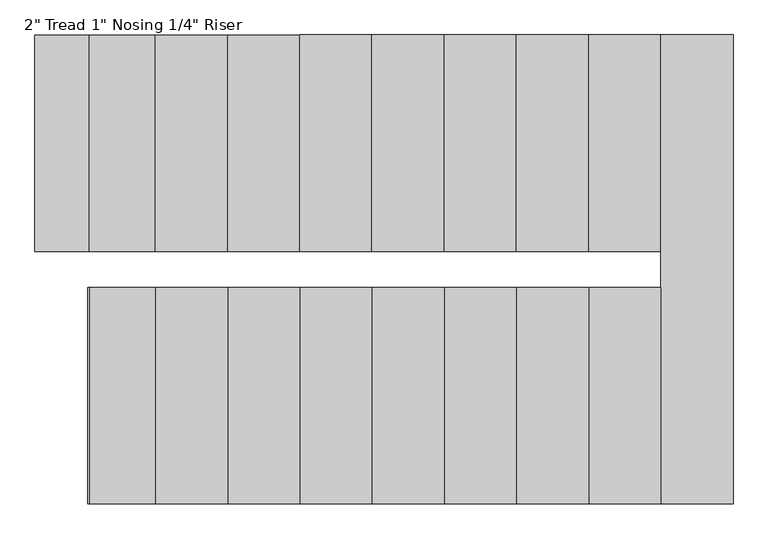
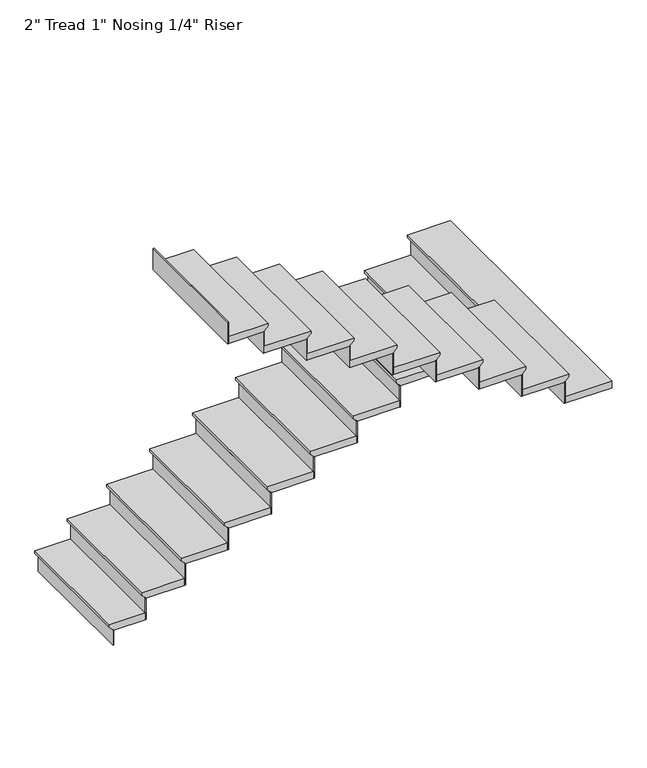
"""IFC4 building model written with IfcOpenShell, lengths in millimetres: stair flight geometry."""

from ifc_helpers import new_model, si_unit, origin, place, context, project, spatial, faceted_brep, source, transform, mapped, element, save


def stair_flight_cd99e03c(model_context):
    return source(origin(), model_context, "Body", "Brep", [
        faceted_brep([(8572.5, 8280.4, 9285.3710526), (8572.5, 8280.4, 9304.4210526), (8572.5, 9194.8, 9304.4210526), (8572.5, 9194.8, 9285.3710526), (8597.9, 8280.4, 9259.9710526), (8597.9, 9194.8, 9259.9710526), (8826.5, 8280.4, 9304.4210526), (8826.5, 9194.8, 9304.4210526), (8597.9, 9194.8, 9253.6210526), (8826.5, 9194.8, 9253.6210526), (8826.5, 8280.4, 9253.6210526), (8597.9, 8280.4, 9253.6210526)], [[[0, 1, 2, 3]], [[4, 0, 3, 5]], [[2, 1, 6, 7]], [[8, 9, 10, 11]], [[2, 7, 9, 8, 5, 3]], [[8, 11, 4, 5]], [[6, 1, 0, 4, 11, 10]], [[7, 6, 10, 9]]]),
        faceted_brep([(8597.9, 8280.4, 9253.6210526), (8597.9, 8280.4, 9144.0), (8604.25, 8280.4, 9144.0), (8604.25, 8280.4, 9253.6210526), (8597.9, 9194.8, 9253.6210526), (8604.25, 9194.8, 9253.6210526), (8604.25, 9194.8, 9144.0), (8597.9, 9194.8, 9144.0)], [[[0, 1, 2, 3]], [[4, 5, 6, 7]], [[1, 0, 4, 7]], [[2, 1, 7, 6]], [[3, 2, 6, 5]], [[0, 3, 5, 4]]]),
        faceted_brep([(8826.5, 8280.4, 9414.0421053), (8826.5, 8280.4, 9253.6210526), (8832.85, 8280.4, 9253.6210526), (8832.85, 8280.4, 9414.0421053), (8826.5, 9194.8, 9414.0421053), (8832.85, 9194.8, 9414.0421053), (8832.85, 9194.8, 9253.6210526), (8826.5, 9194.8, 9253.6210526)], [[[0, 1, 2, 3]], [[4, 5, 6, 7]], [[1, 0, 4, 7]], [[2, 1, 7, 6]], [[3, 2, 6, 5]], [[0, 3, 5, 4]]]),
        faceted_brep([(8801.1, 9194.8, 9464.8421053), (8801.1, 8280.4, 9464.8421053), (9105.9, 8280.4, 9464.8421053), (9105.9, 9194.8, 9464.8421053), (8826.5, 9194.8, 9414.0421053), (9105.9, 9194.8, 9414.0421053), (9105.9, 8280.4, 9414.0421053), (8826.5, 8280.4, 9414.0421053), (8826.5, 9194.8, 9420.3921053), (8801.1, 9194.8, 9445.7921053), (8826.5, 8280.4, 9420.3921053), (8801.1, 8280.4, 9445.7921053)], [[[0, 1, 2, 3]], [[4, 5, 6, 7]], [[0, 3, 5, 4, 8, 9]], [[4, 7, 10, 8]], [[2, 1, 11, 10, 7, 6]], [[3, 2, 6, 5]], [[11, 1, 0, 9]], [[10, 11, 9, 8]]]),
        faceted_brep([(9105.9, 8280.4, 9574.4631579), (9105.9, 8280.4, 9414.0421053), (9112.25, 8280.4, 9414.0421053), (9112.25, 8280.4, 9574.4631579), (9105.9, 9194.8, 9574.4631579), (9112.25, 9194.8, 9574.4631579), (9112.25, 9194.8, 9414.0421053), (9105.9, 9194.8, 9414.0421053)], [[[0, 1, 2, 3]], [[4, 5, 6, 7]], [[1, 0, 4, 7]], [[2, 1, 7, 6]], [[3, 2, 6, 5]], [[0, 3, 5, 4]]]),
        faceted_brep([(9080.5, 9194.8, 9625.2631579), (9080.5, 8280.4, 9625.2631579), (9410.7, 8280.4, 9625.2631579), (9410.7, 9194.8, 9625.2631579), (9105.9, 9194.8, 9574.4631579), (9410.7, 9194.8, 9574.4631579), (9410.7, 8280.4, 9574.4631579), (9105.9, 8280.4, 9574.4631579), (9105.9, 9194.8, 9580.8131579), (9080.5, 9194.8, 9606.2131579), (9105.9, 8280.4, 9580.8131579), (9080.5, 8280.4, 9606.2131579)], [[[0, 1, 2, 3]], [[4, 5, 6, 7]], [[0, 3, 5, 4, 8, 9]], [[4, 7, 10, 8]], [[2, 1, 11, 10, 7, 6]], [[3, 2, 6, 5]], [[11, 1, 0, 9]], [[10, 11, 9, 8]]]),
        faceted_brep([(9410.7, 8280.4, 9734.8842105), (9410.7, 8280.4, 9574.4631579), (9417.05, 8280.4, 9574.4631579), (9417.05, 8280.4, 9734.8842105), (9410.7, 9194.8, 9734.8842105), (9417.05, 9194.8, 9734.8842105), (9417.05, 9194.8, 9574.4631579), (9410.7, 9194.8, 9574.4631579)], [[[0, 1, 2, 3]], [[4, 5, 6, 7]], [[1, 0, 4, 7]], [[2, 1, 7, 6]], [[3, 2, 6, 5]], [[0, 3, 5, 4]]]),
        faceted_brep([(9385.3, 9194.8, 9785.6842105), (9385.3, 8280.4, 9785.6842105), (9715.5, 8280.4, 9785.6842105), (9715.5, 9194.8, 9785.6842105), (9410.7, 9194.8, 9734.8842105), (9715.5, 9194.8, 9734.8842105), (9715.5, 8280.4, 9734.8842105), (9410.7, 8280.4, 9734.8842105), (9410.7, 9194.8, 9741.2342105), (9385.3, 9194.8, 9766.6342105), (9410.7, 8280.4, 9741.2342105), (9385.3, 8280.4, 9766.6342105)], [[[0, 1, 2, 3]], [[4, 5, 6, 7]], [[0, 3, 5, 4, 8, 9]], [[4, 7, 10, 8]], [[2, 1, 11, 10, 7, 6]], [[3, 2, 6, 5]], [[11, 1, 0, 9]], [[10, 11, 9, 8]]]),
        faceted_brep([(9715.5, 8280.4, 9895.3052632), (9715.5, 8280.4, 9734.8842105), (9721.85, 8280.4, 9734.8842105), (9721.85, 8280.4, 9895.3052632), (9715.5, 9194.8, 9895.3052632), (9721.85, 9194.8, 9895.3052632), (9721.85, 9194.8, 9734.8842105), (9715.5, 9194.8, 9734.8842105)], [[[0, 1, 2, 3]], [[4, 5, 6, 7]], [[1, 0, 4, 7]], [[2, 1, 7, 6]], [[3, 2, 6, 5]], [[0, 3, 5, 4]]]),
        faceted_brep([(9690.1, 9194.8, 9946.1052632), (9690.1, 8280.4, 9946.1052632), (10020.3, 8280.4, 9946.1052632), (10020.3, 9194.8, 9946.1052632), (9715.5, 9194.8, 9895.3052632), (10020.3, 9194.8, 9895.3052632), (10020.3, 8280.4, 9895.3052632), (9715.5, 8280.4, 9895.3052632), (9715.5, 9194.8, 9901.6552632), (9690.1, 9194.8, 9927.0552632), (9715.5, 8280.4, 9901.6552632), (9690.1, 8280.4, 9927.0552632)], [[[0, 1, 2, 3]], [[4, 5, 6, 7]], [[0, 3, 5, 4, 8, 9]], [[4, 7, 10, 8]], [[2, 1, 11, 10, 7, 6]], [[3, 2, 6, 5]], [[11, 1, 0, 9]], [[10, 11, 9, 8]]]),
        faceted_brep([(10020.3, 8280.4, 10055.7263158), (10020.3, 8280.4, 9895.3052632), (10026.65, 8280.4, 9895.3052632), (10026.65, 8280.4, 10055.7263158), (10020.3, 9194.8, 10055.7263158), (10026.65, 9194.8, 10055.7263158), (10026.65, 9194.8, 9895.3052632), (10020.3, 9194.8, 9895.3052632)], [[[0, 1, 2, 3]], [[4, 5, 6, 7]], [[1, 0, 4, 7]], [[2, 1, 7, 6]], [[3, 2, 6, 5]], [[0, 3, 5, 4]]]),
        faceted_brep([(9994.9, 9194.8, 10106.5263158), (9994.9, 8280.4, 10106.5263158), (10325.1, 8280.4, 10106.5263158), (10325.1, 9194.8, 10106.5263158), (10020.3, 9194.8, 10055.7263158), (10325.1, 9194.8, 10055.7263158), (10325.1, 8280.4, 10055.7263158), (10020.3, 8280.4, 10055.7263158), (10020.3, 9194.8, 10062.0763158), (9994.9, 9194.8, 10087.4763158), (10020.3, 8280.4, 10062.0763158), (9994.9, 8280.4, 10087.4763158)], [[[0, 1, 2, 3]], [[4, 5, 6, 7]], [[0, 3, 5, 4, 8, 9]], [[4, 7, 10, 8]], [[2, 1, 11, 10, 7, 6]], [[3, 2, 6, 5]], [[11, 1, 0, 9]], [[10, 11, 9, 8]]]),
        faceted_brep([(10325.1, 8280.4, 10216.1473684), (10325.1, 8280.4, 10055.7263158), (10331.45, 8280.4, 10055.7263158), (10331.45, 8280.4, 10216.1473684), (10325.1, 9194.8, 10216.1473684), (10331.45, 9194.8, 10216.1473684), (10331.45, 9194.8, 10055.7263158), (10325.1, 9194.8, 10055.7263158)], [[[0, 1, 2, 3]], [[4, 5, 6, 7]], [[1, 0, 4, 7]], [[2, 1, 7, 6]], [[3, 2, 6, 5]], [[0, 3, 5, 4]]]),
        faceted_brep([(10299.7, 9194.8, 10266.9473684), (10299.7, 8280.4, 10266.9473684), (10629.9, 8280.4, 10266.9473684), (10629.9, 9194.8, 10266.9473684), (10325.1, 9194.8, 10216.1473684), (10629.9, 9194.8, 10216.1473684), (10629.9, 8280.4, 10216.1473684), (10325.1, 8280.4, 10216.1473684), (10325.1, 9194.8, 10222.4973684), (10299.7, 9194.8, 10247.8973684), (10325.1, 8280.4, 10222.4973684), (10299.7, 8280.4, 10247.8973684)], [[[0, 1, 2, 3]], [[4, 5, 6, 7]], [[0, 3, 5, 4, 8, 9]], [[4, 7, 10, 8]], [[2, 1, 11, 10, 7, 6]], [[3, 2, 6, 5]], [[11, 1, 0, 9]], [[10, 11, 9, 8]]]),
        faceted_brep([(10629.9, 8280.4, 10376.5684211), (10629.9, 8280.4, 10216.1473684), (10636.25, 8280.4, 10216.1473684), (10636.25, 8280.4, 10376.5684211), (10629.9, 9194.8, 10376.5684211), (10636.25, 9194.8, 10376.5684211), (10636.25, 9194.8, 10216.1473684), (10629.9, 9194.8, 10216.1473684)], [[[0, 1, 2, 3]], [[4, 5, 6, 7]], [[1, 0, 4, 7]], [[2, 1, 7, 6]], [[3, 2, 6, 5]], [[0, 3, 5, 4]]]),
        faceted_brep([(10604.5, 9194.8, 10427.3684211), (10604.5, 8280.4, 10427.3684211), (10934.7, 8280.4, 10427.3684211), (10934.7, 9194.8, 10427.3684211), (10629.9, 9194.8, 10376.5684211), (10934.7, 9194.8, 10376.5684211), (10934.7, 8280.4, 10376.5684211), (10629.9, 8280.4, 10376.5684211), (10629.9, 9194.8, 10382.9184211), (10604.5, 9194.8, 10408.3184211), (10629.9, 8280.4, 10382.9184211), (10604.5, 8280.4, 10408.3184211)], [[[0, 1, 2, 3]], [[4, 5, 6, 7]], [[0, 3, 5, 4, 8, 9]], [[4, 7, 10, 8]], [[2, 1, 11, 10, 7, 6]], [[3, 2, 6, 5]], [[11, 1, 0, 9]], [[10, 11, 9, 8]]]),
        faceted_brep([(10934.7, 8280.4, 10536.9894737), (10934.7, 8280.4, 10376.5684211), (10941.05, 8280.4, 10376.5684211), (10941.05, 8280.4, 10536.9894737), (10934.7, 9194.8, 10536.9894737), (10941.05, 9194.8, 10536.9894737), (10941.05, 9194.8, 10376.5684211), (10934.7, 9194.8, 10376.5684211)], [[[0, 1, 2, 3]], [[4, 5, 6, 7]], [[1, 0, 4, 7]], [[2, 1, 7, 6]], [[3, 2, 6, 5]], [[0, 3, 5, 4]]]),
        faceted_brep([(10909.3, 9194.8, 10587.7894737), (10909.3, 8280.4, 10587.7894737), (11239.5, 8280.4, 10587.7894737), (11239.5, 9194.8, 10587.7894737), (10934.7, 9194.8, 10536.9894737), (11239.5, 9194.8, 10536.9894737), (11239.5, 8280.4, 10536.9894737), (10934.7, 8280.4, 10536.9894737), (10934.7, 9194.8, 10543.3394737), (10909.3, 9194.8, 10568.7394737), (10934.7, 8280.4, 10543.3394737), (10909.3, 8280.4, 10568.7394737)], [[[0, 1, 2, 3]], [[4, 5, 6, 7]], [[0, 3, 5, 4, 8, 9]], [[4, 7, 10, 8]], [[2, 1, 11, 10, 7, 6]], [[3, 2, 6, 5]], [[11, 1, 0, 9]], [[10, 11, 9, 8]]]),
        faceted_brep([(11239.5, 8280.4, 10697.4105263), (11239.5, 8280.4, 10536.9894737), (11245.85, 8280.4, 10536.9894737), (11245.85, 8280.4, 10697.4105263), (11239.5, 9194.8, 10697.4105263), (11245.85, 9194.8, 10697.4105263), (11245.85, 9194.8, 10536.9894737), (11239.5, 9194.8, 10536.9894737)], [[[0, 1, 2, 3]], [[4, 5, 6, 7]], [[1, 0, 4, 7]], [[2, 1, 7, 6]], [[3, 2, 6, 5]], [[0, 3, 5, 4]]]),
        faceted_brep([(11188.7, 7213.6, 10748.2105263), (11518.9, 7213.6, 10748.2105263), (11518.9, 9194.8, 10748.2105263), (11214.1, 9194.8, 10748.2105263), (11214.1, 8128.0, 10748.2105263), (11188.7, 8128.0, 10748.2105263), (11518.9, 7213.6, 10697.4105263), (11188.7, 7213.6, 10697.4105263), (11188.7, 8128.0, 10697.4105263), (11214.1, 8128.0, 10697.4105263), (11214.1, 8280.4, 10697.4105263), (11239.5, 8280.4, 10697.4105263), (11239.5, 9194.8, 10697.4105263), (11518.9, 9194.8, 10697.4105263), (11239.5, 9194.8, 10703.7605263), (11214.1, 9194.8, 10729.1605263), (11239.5, 8280.4, 10703.7605263), (11214.1, 8280.4, 10729.1605263)], [[[0, 1, 2, 3, 4, 5]], [[6, 7, 8, 9, 10, 11, 12, 13]], [[1, 0, 7, 6]], [[2, 1, 6, 13]], [[3, 2, 13, 12, 14, 15]], [[12, 11, 16, 14]], [[11, 10, 17, 16]], [[4, 3, 15, 17, 10, 9]], [[5, 4, 9, 8]], [[0, 5, 8, 7]], [[15, 14, 16, 17]]]),
        faceted_brep([(11188.7, 8128.0, 10857.8315789), (11188.7, 8128.0, 10697.4105263), (11182.35, 8128.0, 10697.4105263), (11182.35, 8128.0, 10857.8315789), (11188.7, 7213.6, 10857.8315789), (11182.35, 7213.6, 10857.8315789), (11182.35, 7213.6, 10697.4105263), (11188.7, 7213.6, 10697.4105263)], [[[0, 1, 2, 3]], [[4, 5, 6, 7]], [[1, 0, 4, 7]], [[2, 1, 7, 6]], [[3, 2, 6, 5]], [[0, 3, 5, 4]]]),
        faceted_brep([(11214.1, 7213.6, 10908.6315789), (11214.1, 8128.0, 10908.6315789), (10883.9, 8128.0, 10908.6315789), (10883.9, 7213.6, 10908.6315789), (11188.7, 7213.6, 10857.8315789), (10883.9, 7213.6, 10857.8315789), (10883.9, 8128.0, 10857.8315789), (11188.7, 8128.0, 10857.8315789), (11188.7, 7213.6, 10864.1815789), (11214.1, 7213.6, 10889.5815789), (11188.7, 8128.0, 10864.1815789), (11214.1, 8128.0, 10889.5815789)], [[[0, 1, 2, 3]], [[4, 5, 6, 7]], [[0, 3, 5, 4, 8, 9]], [[4, 7, 10, 8]], [[2, 1, 11, 10, 7, 6]], [[3, 2, 6, 5]], [[11, 1, 0, 9]], [[10, 11, 9, 8]]]),
        faceted_brep([(10883.9, 8128.0, 11018.2526316), (10883.9, 8128.0, 10857.8315789), (10877.55, 8128.0, 10857.8315789), (10877.55, 8128.0, 11018.2526316), (10883.9, 7213.6, 11018.2526316), (10877.55, 7213.6, 11018.2526316), (10877.55, 7213.6, 10857.8315789), (10883.9, 7213.6, 10857.8315789)], [[[0, 1, 2, 3]], [[4, 5, 6, 7]], [[1, 0, 4, 7]], [[2, 1, 7, 6]], [[3, 2, 6, 5]], [[0, 3, 5, 4]]]),
        faceted_brep([(10909.3, 7213.6, 11069.0526316), (10909.3, 8128.0, 11069.0526316), (10579.1, 8128.0, 11069.0526316), (10579.1, 7213.6, 11069.0526316), (10883.9, 7213.6, 11018.2526316), (10579.1, 7213.6, 11018.2526316), (10579.1, 8128.0, 11018.2526316), (10883.9, 8128.0, 11018.2526316), (10883.9, 7213.6, 11024.6026316), (10909.3, 7213.6, 11050.0026316), (10883.9, 8128.0, 11024.6026316), (10909.3, 8128.0, 11050.0026316)], [[[0, 1, 2, 3]], [[4, 5, 6, 7]], [[0, 3, 5, 4, 8, 9]], [[4, 7, 10, 8]], [[2, 1, 11, 10, 7, 6]], [[3, 2, 6, 5]], [[11, 1, 0, 9]], [[10, 11, 9, 8]]]),
        faceted_brep([(10579.1, 8128.0, 11178.6736842), (10579.1, 8128.0, 11018.2526316), (10572.75, 8128.0, 11018.2526316), (10572.75, 8128.0, 11178.6736842), (10579.1, 7213.6, 11178.6736842), (10572.75, 7213.6, 11178.6736842), (10572.75, 7213.6, 11018.2526316), (10579.1, 7213.6, 11018.2526316)], [[[0, 1, 2, 3]], [[4, 5, 6, 7]], [[1, 0, 4, 7]], [[2, 1, 7, 6]], [[3, 2, 6, 5]], [[0, 3, 5, 4]]]),
        faceted_brep([(10604.5, 7213.6, 11229.4736842), (10604.5, 8128.0, 11229.4736842), (10274.3, 8128.0, 11229.4736842), (10274.3, 7213.6, 11229.4736842), (10579.1, 7213.6, 11178.6736842), (10274.3, 7213.6, 11178.6736842), (10274.3, 8128.0, 11178.6736842), (10579.1, 8128.0, 11178.6736842), (10579.1, 7213.6, 11185.0236842), (10604.5, 7213.6, 11210.4236842), (10579.1, 8128.0, 11185.0236842), (10604.5, 8128.0, 11210.4236842)], [[[0, 1, 2, 3]], [[4, 5, 6, 7]], [[0, 3, 5, 4, 8, 9]], [[4, 7, 10, 8]], [[2, 1, 11, 10, 7, 6]], [[3, 2, 6, 5]], [[11, 1, 0, 9]], [[10, 11, 9, 8]]]),
        faceted_brep([(10274.3, 8128.0, 11339.0947368), (10274.3, 8128.0, 11178.6736842), (10267.95, 8128.0, 11178.6736842), (10267.95, 8128.0, 11339.0947368), (10274.3, 7213.6, 11339.0947368), (10267.95, 7213.6, 11339.0947368), (10267.95, 7213.6, 11178.6736842), (10274.3, 7213.6, 11178.6736842)], [[[0, 1, 2, 3]], [[4, 5, 6, 7]], [[1, 0, 4, 7]], [[2, 1, 7, 6]], [[3, 2, 6, 5]], [[0, 3, 5, 4]]]),
        faceted_brep([(10299.7, 7213.6, 11389.8947368), (10299.7, 8128.0, 11389.8947368), (9969.5, 8128.0, 11389.8947368), (9969.5, 7213.6, 11389.8947368), (10274.3, 7213.6, 11339.0947368), (9969.5, 7213.6, 11339.0947368), (9969.5, 8128.0, 11339.0947368), (10274.3, 8128.0, 11339.0947368), (10274.3, 7213.6, 11345.4447368), (10299.7, 7213.6, 11370.8447368), (10274.3, 8128.0, 11345.4447368), (10299.7, 8128.0, 11370.8447368)], [[[0, 1, 2, 3]], [[4, 5, 6, 7]], [[0, 3, 5, 4, 8, 9]], [[4, 7, 10, 8]], [[2, 1, 11, 10, 7, 6]], [[3, 2, 6, 5]], [[11, 1, 0, 9]], [[10, 11, 9, 8]]]),
        faceted_brep([(9969.5, 8128.0, 11499.5157895), (9969.5, 8128.0, 11339.0947368), (9963.15, 8128.0, 11339.0947368), (9963.15, 8128.0, 11499.5157895), (9969.5, 7213.6, 11499.5157895), (9963.15, 7213.6, 11499.5157895), (9963.15, 7213.6, 11339.0947368), (9969.5, 7213.6, 11339.0947368)], [[[0, 1, 2, 3]], [[4, 5, 6, 7]], [[1, 0, 4, 7]], [[2, 1, 7, 6]], [[3, 2, 6, 5]], [[0, 3, 5, 4]]]),
        faceted_brep([(9994.9, 7213.6, 11550.3157895), (9994.9, 8128.0, 11550.3157895), (9664.7, 8128.0, 11550.3157895), (9664.7, 7213.6, 11550.3157895), (9969.5, 7213.6, 11499.5157895), (9664.7, 7213.6, 11499.5157895), (9664.7, 8128.0, 11499.5157895), (9969.5, 8128.0, 11499.5157895), (9969.5, 7213.6, 11505.8657895), (9994.9, 7213.6, 11531.2657895), (9969.5, 8128.0, 11505.8657895), (9994.9, 8128.0, 11531.2657895)], [[[0, 1, 2, 3]], [[4, 5, 6, 7]], [[0, 3, 5, 4, 8, 9]], [[4, 7, 10, 8]], [[2, 1, 11, 10, 7, 6]], [[3, 2, 6, 5]], [[11, 1, 0, 9]], [[10, 11, 9, 8]]]),
        faceted_brep([(9664.7, 8128.0, 11659.9368421), (9664.7, 8128.0, 11499.5157895), (9658.35, 8128.0, 11499.5157895), (9658.35, 8128.0, 11659.9368421), (9664.7, 7213.6, 11659.9368421), (9658.35, 7213.6, 11659.9368421), (9658.35, 7213.6, 11499.5157895), (9664.7, 7213.6, 11499.5157895)], [[[0, 1, 2, 3]], [[4, 5, 6, 7]], [[1, 0, 4, 7]], [[2, 1, 7, 6]], [[3, 2, 6, 5]], [[0, 3, 5, 4]]]),
        faceted_brep([(9690.1, 7213.6, 11710.7368421), (9690.1, 8128.0, 11710.7368421), (9359.9, 8128.0, 11710.7368421), (9359.9, 7213.6, 11710.7368421), (9664.7, 7213.6, 11659.9368421), (9359.9, 7213.6, 11659.9368421), (9359.9, 8128.0, 11659.9368421), (9664.7, 8128.0, 11659.9368421), (9664.7, 7213.6, 11666.2868421), (9690.1, 7213.6, 11691.6868421), (9664.7, 8128.0, 11666.2868421), (9690.1, 8128.0, 11691.6868421)], [[[0, 1, 2, 3]], [[4, 5, 6, 7]], [[0, 3, 5, 4, 8, 9]], [[4, 7, 10, 8]], [[2, 1, 11, 10, 7, 6]], [[3, 2, 6, 5]], [[11, 1, 0, 9]], [[10, 11, 9, 8]]]),
        faceted_brep([(9359.9, 8128.0, 11820.3578947), (9359.9, 8128.0, 11659.9368421), (9353.55, 8128.0, 11659.9368421), (9353.55, 8128.0, 11820.3578947), (9359.9, 7213.6, 11820.3578947), (9353.55, 7213.6, 11820.3578947), (9353.55, 7213.6, 11659.9368421), (9359.9, 7213.6, 11659.9368421)], [[[0, 1, 2, 3]], [[4, 5, 6, 7]], [[1, 0, 4, 7]], [[2, 1, 7, 6]], [[3, 2, 6, 5]], [[0, 3, 5, 4]]]),
        faceted_brep([(9385.3, 7213.6, 11871.1578947), (9385.3, 8128.0, 11871.1578947), (9055.1, 8128.0, 11871.1578947), (9055.1, 7213.6, 11871.1578947), (9359.9, 7213.6, 11820.3578947), (9055.1, 7213.6, 11820.3578947), (9055.1, 8128.0, 11820.3578947), (9359.9, 8128.0, 11820.3578947), (9359.9, 7213.6, 11826.7078947), (9385.3, 7213.6, 11852.1078947), (9359.9, 8128.0, 11826.7078947), (9385.3, 8128.0, 11852.1078947)], [[[0, 1, 2, 3]], [[4, 5, 6, 7]], [[0, 3, 5, 4, 8, 9]], [[4, 7, 10, 8]], [[2, 1, 11, 10, 7, 6]], [[3, 2, 6, 5]], [[11, 1, 0, 9]], [[10, 11, 9, 8]]]),
        faceted_brep([(9055.1, 8128.0, 11980.7789474), (9055.1, 8128.0, 11820.3578947), (9048.75, 8128.0, 11820.3578947), (9048.75, 8128.0, 11980.7789474), (9055.1, 7213.6, 11980.7789474), (9048.75, 7213.6, 11980.7789474), (9048.75, 7213.6, 11820.3578947), (9055.1, 7213.6, 11820.3578947)], [[[0, 1, 2, 3]], [[4, 5, 6, 7]], [[1, 0, 4, 7]], [[2, 1, 7, 6]], [[3, 2, 6, 5]], [[0, 3, 5, 4]]]),
        faceted_brep([(8801.1, 8128.0, 12141.2), (8801.1, 8128.0, 11980.7789474), (8794.75, 8128.0, 11980.7789474), (8794.75, 8128.0, 12141.2), (8801.1, 7213.6, 12141.2), (8794.75, 7213.6, 12141.2), (8794.75, 7213.6, 11980.7789474), (8801.1, 7213.6, 11980.7789474)], [[[0, 1, 2, 3]], [[4, 5, 6, 7]], [[1, 0, 4, 7]], [[2, 1, 7, 6]], [[3, 2, 6, 5]], [[0, 3, 5, 4]]]),
        faceted_brep([(9080.5, 7213.6, 12031.5789474), (9080.5, 8128.0, 12031.5789474), (8801.1, 8128.0, 12031.5789474), (8801.1, 7213.6, 12031.5789474), (9055.1, 7213.6, 11980.7789474), (8801.1, 7213.6, 11980.7789474), (8801.1, 8128.0, 11980.7789474), (9055.1, 8128.0, 11980.7789474), (9055.1, 7213.6, 11987.1289474), (9080.5, 7213.6, 12012.5289474), (9055.1, 8128.0, 11987.1289474), (9080.5, 8128.0, 12012.5289474)], [[[0, 1, 2, 3]], [[4, 5, 6, 7]], [[0, 3, 5, 4, 8, 9]], [[4, 7, 10, 8]], [[2, 1, 11, 10, 7, 6]], [[3, 2, 6, 5]], [[11, 1, 0, 9]], [[10, 11, 9, 8]]]),
    ])


if __name__ == "__main__":
    model = new_model("IFC4")
    model_context = context("Model", 3, world=origin())
    ifc_project = project(units=[si_unit("LENGTHUNIT", "METRE", prefix="MILLI")], contexts=[model_context])
    site = spatial("IfcSite", under=ifc_project)
    building = spatial("IfcBuilding", under=site)
    placement = place(None, origin())
    stair_flight_shape = stair_flight_cd99e03c(model_context)
    element("IfcStairFlight", 1, ObjectType="2\" Tread 1\" Nosing 1/4\" Riser", at=placement, inside=building, context=model_context, shape_type="MappedRepresentation", body=[
        mapped(stair_flight_shape, transform((0.0, 0.0, 0.0), x_axis=(1.0, 0.0, 0.0), y_axis=(0.0, 1.0, 0.0), z_axis=(0.0, 0.0, 1.0))),
    ])
    save(model, "model.ifc")
